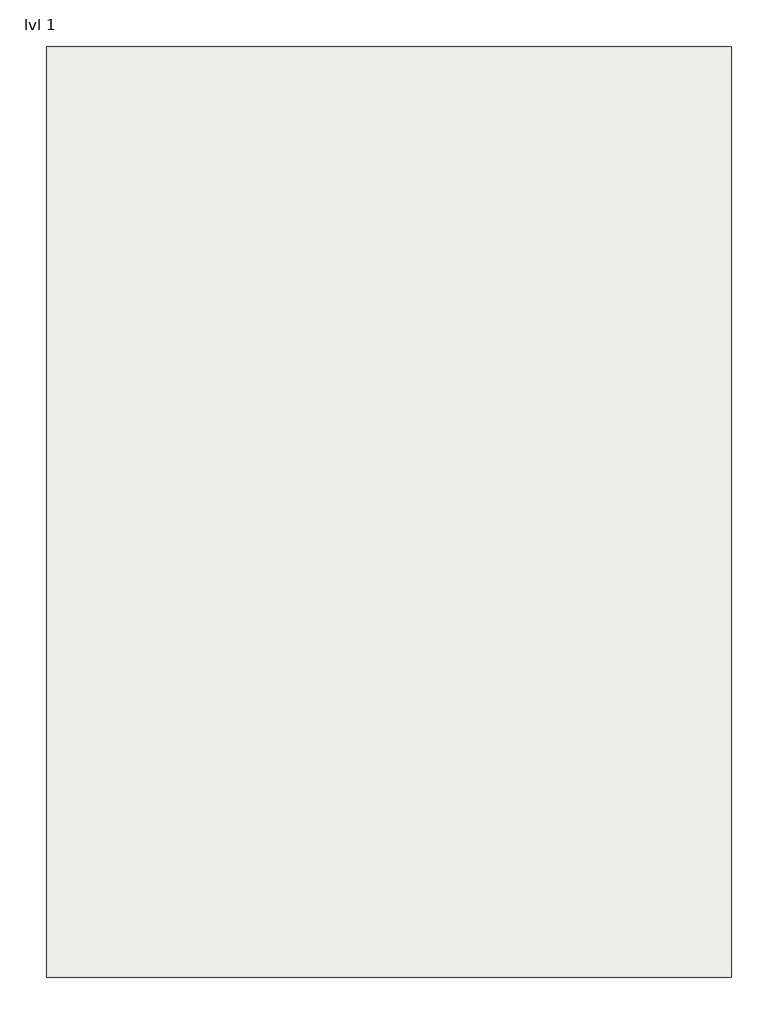
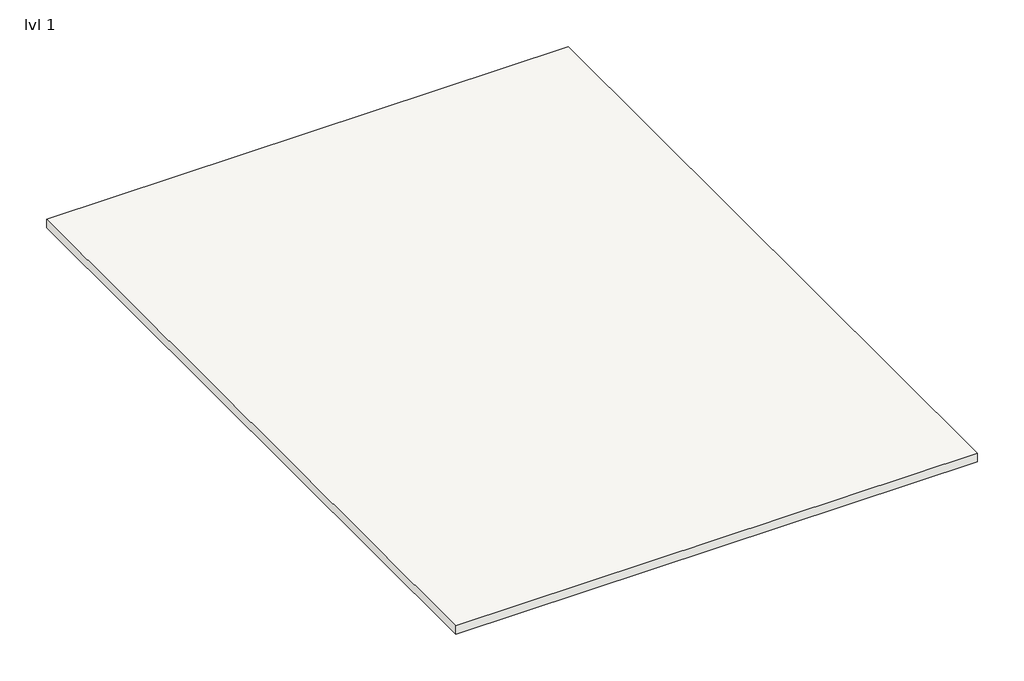
# One storey: 1 roof.
"""IFC4 building model written with IfcOpenShell, lengths in millimetres."""

from ifc_helpers import new_model, si_unit, frame, origin, place, context, project, spatial, polyline, outline, extrude, element, save

model = new_model("IFC4")

# Units and contexts
model_context = context("Model", 3, world=origin())
ifc_project = project(units=[si_unit("LENGTHUNIT", "METRE", prefix="MILLI")], contexts=[model_context])

# Site, building, storey
site = spatial("IfcSite", under=ifc_project)
building = spatial("IfcBuilding", under=site)
storey = spatial("IfcBuildingStorey", under=building, Name="lvl 1", Elevation=3048.0)

# Roof
placement = place(None, origin())
element("IfcRoof", 1, ObjectType="6\" slab", at=placement, inside=storey, context=model_context, shape_type="SweptSolid", body=[
    extrude(outline(polyline([(-22919.6899593, 8118.7908098), (-14004.2899593, 8118.7908098), (-14004.2899593, -3997.0091902), (-22919.6899593, -3997.0091902), (-22919.6899593, 8118.7908098)])), frame((0.0, 0.0, 3048.0), z_axis=(0.0, 0.0, 1.0), x_axis=(1.0, 0.0, 0.0)), (0.0, 0.0, 1.0), 152.4),
])

save(model, "model.ifc")

# Revit data of these elements
# Type "6\" slab"
#   Assembly Code = "B1020"
#   Layers, outside or top first: 0' - 6" no material (function 1)
# Element 1 (IfcRoof, "6\" slab")
#   built-in parameter 1001705 = 10.5 (stored number, unit not read)
#   built-in parameter 1001710 = 33615
#   Phase Created = New Construction
#   Materials on its faces: "Default Roof"
# Materials
#   "Default Roof": colour RGB 88 101 114, transparency 0, Cost = 0
